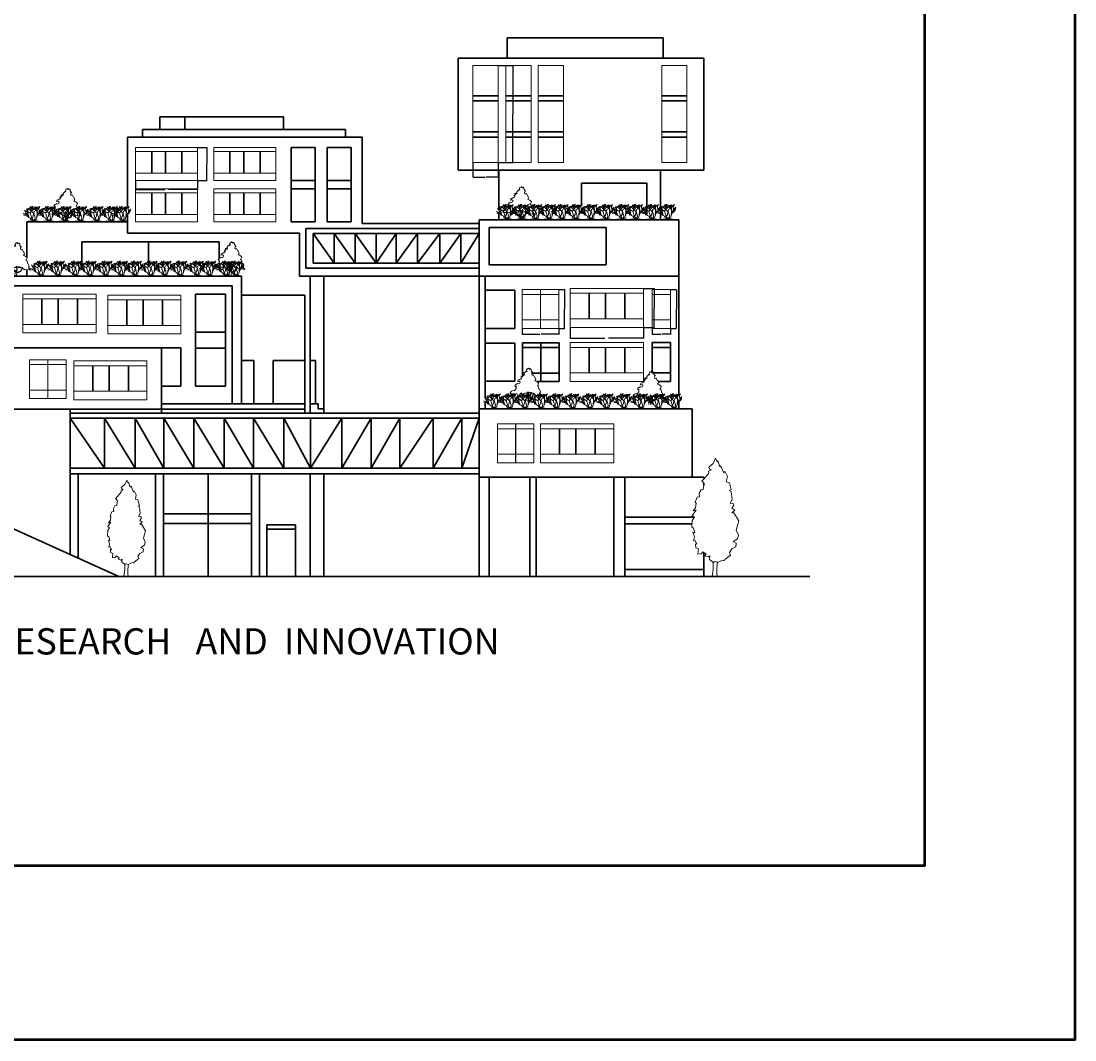
# Model space of a CAD drawing. Units: inches. Extents: x -1080 to 1950, y -1929 to 857.
# Tile 7 of 16: x 991 to 1950, y -1929 to -1001. Entities that reach past the tile are written whole.
import ezdxf

# ---------------------------------------------------------------- set-up
doc = ezdxf.new("R2010")
doc.units = ezdxf.units.IN
doc.header["$MEASUREMENT"] = 0
for name, color, linetype, lineweight in [('A-ANNO-DIMS', 2, 'Continuous', 18), ('A-ANNO-TEXT', 7, 'Continuous', 25), ('A-ANNO-TTLB', 7, 'Continuous', 50), ('A-ELEV', 7, 'Continuous', 35), ('A-GLAZ', 4, 'Continuous', 18), ('L-PLNT', 82, 'Continuous', 13)]:
    doc.layers.add(name, color=color, linetype=linetype, lineweight=lineweight)
doc.styles.get("Standard").update_dxf_attribs({"font": 'arial.ttf'})
doc.dimstyles.get("Standard").update_dxf_attribs({"dimtxt": 0.18, "dimasz": 0.18, "dimexe": 0.18, "dimexo": 0.0625, "dimgap": 0.09, "dimtad": 0, "dimtih": 1, "dimtoh": 1, "dimdec": 4, "dimzin": 0, "dimdsep": 46, "dimtxsty": 'Standard', "dimcen": 0.09, "dimadec": 0, "dimazin": 0, "dimtfac": 1, "dimtdec": 4, "dimtofl": 0, "dimtmove": 0, "dimatfit": 3, "dimfxl": 1, "dimtolj": 1, "dimtzin": 0, "dimarcsym": 0})

# ---------------------------------------------------------------- blocks, each defined once
blk = doc.blocks.new('*U5')
blk.add_lwpolyline([(-2.754, 191.699), (-6.78, 182.851), (-13.682, 176.953), (-11.956, 173.266), (-9.656, 172.529), (-14.257, 170.317), (-13.682, 167.368), (-21.733, 157.783), (-25.184, 154.834), (-21.158, 150.41), (-21.733, 147.461), (-22.884, 140.825), (-26.334, 140.087), (-29.21, 134.926), (-28.635, 129.028), (-32.661, 128.291), (-36.111, 120.18), (-34.386, 118.706), (-35.536, 111.333), (-38.987, 106.171), (-34.386, 107.646), (-40.712, 98.798), (-37.261, 95.849), (-40.712, 90.688), (-41.287, 80.366), (-38.412, 78.154), (-36.686, 70.781), (-39.562, 71.518), (-37.261, 64.145), (-38.412, 57.509), (-36.111, 58.247), (-33.236, 52.348), (-35.536, 53.086), (-34.961, 46.45), (-30.36, 44.975), (-31.51, 36.128), (-26.334, 36.865), (-23.459, 39.814), (-18.283, 36.128), (-20.008, 33.178), (-14.832, 31.704), (-11.956, 33.178), (-12.531, 27.28), (-6.205, 22.856), (-3.905, 24.331), (0.121, 22.856), (8.173, 26.543), (11.624, 25.068), (12.199, 27.28), (21.4, 34.653), (19.675, 39.077), (23.701, 44.975), (30.027, 47.924), (30.602, 53.823), (25.426, 56.772), (32.903, 61.196), (34.053, 67.094), (30.602, 75.205), (34.628, 89.951), (26.576, 103.222), (23.701, 103.222), (28.302, 107.646), (23.701, 110.595), (26.576, 115.756), (25.426, 117.968), (20.825, 118.706), (24.276, 124.604), (22.551, 137.876), (19.1, 139.35), (22.551, 140.825), (19.675, 151.884), (14.499, 153.359), (16.224, 162.207), (12.199, 170.317), (10.473, 167.368), (5.872, 179.165), (4.147, 177.69), (0.696, 187.275), (-0.454, 185.8)], close=True)
for points in [[(-6.813, 23.669), (-6.813, 11.669), (-8.627, 0)], [(0.387, 23.669), (-0.576, 13.271), (-0.576, 3.686), (0, 0)]]:
    blk.add_lwpolyline(points)
blk = doc.blocks.new('*U2')
for points in [[(22.0124, 137.721), (18.5475, 141.5624), (15.5282, 138.2446), (13.8028, 139.3505), (13.3714, 142.1153), (11.2148, 143.2214), (8.1954, 140.4564), (4.7447, 141.0094), (2.1567, 136.0326), (2.1567, 131.6088), (5.6074, 129.9499), (3.0193, 128.2909), (0.4313, 130.5029), (-6.9015, 123.3141), (-6.9015, 121.6552), (-9.9208, 119.9963), (-9.0581, 118.3373), (-6.9015, 115.0195), (-10.7835, 112.2546), (-14.6656, 115.0195), (-16.8222, 114.4665), (-17.6849, 112.2546), (-14.6656, 111.7016), (-14.2342, 107.2778), (-17.6065, 107.8307), (-21.5669, 103.9599), (-17.2536, 103.4069), (-18.9789, 97.8771), (-22.8609, 97.3241), (-27.1743, 94.5593), (-32.3504, 91.7944), (-32.7817, 94.0063), (-36.6638, 85.7116), (-29.7624, 87.3705), (-25.449, 84.6056), (-26.743, 77.9699), (-34.507, 75.205), (-37.9578, 77.4169), (-39.2518, 74.099), (-42.2711, 73.5461), (-44.8592, 70.2282), (-47.8786, 66.3574), (-43.9965, 63.0395), (-41.4085, 64.6985), (-44.3346, 59.8898), (-42.2089, 60.1377), (-42.5159, 55.7849), (-49.6039, 46.4502), (-58.2307, 45.8972), (-62.1127, 43.6853), (-68.5828, 36.4966), (-65.9947, 32.0727), (-50.0352, 32.6257), (-47.0159, 30.4138), (-39.6831, 33.7317), (-34.507, 22.6721), (-32.3504, 22.6721), (-22.4296, 34.8376), (-19.4102, 36.4966), (-17.2536, 33.7317), (-17.2536, 29.8608), (-13.8028, 28.7549), (-9.0581, 28.7549), (-7.3328, 32.6257), (-1.7254, 35.3906), (3.8821, 35.9436), (6.4701, 38.1555), (6.9014, 38.7085), (8.1954, 41.4734), (9.9208, 40.3674), (11.2148, 35.9436), (14.2341, 37.6025), (15.0968, 36.4966), (15.9595, 33.7317), (18.9789, 38.7085), (21.9982, 38.7085), (23.2922, 36.4966), (21.9982, 34.2847), (25.4489, 35.3906), (26.743, 33.7317), (29.7623, 35.9436), (32.7817, 34.8376), (38.8204, 28.7549), (41.4084, 27.6489), (43.5651, 25.437), (61.6813, 27.0959), (65.132, 23.7781), (67.7201, 24.884), (60.8186, 33.7317), (60.3873, 37.0495), (62.544, 40.3674), (58.662, 50.874), (56.5053, 50.874), (52.1919, 66.3574), (47.8785, 66.9103), (50.4665, 69.1222), (53.9172, 77.9699), (47.0158, 85.1586), (38.3891, 87.9235), (42.2711, 94.0063)], [(42.2711, 94.0063), (38.8204, 104.5129), (36.6637, 104.5129), (32.3503, 113.9135), (29.7623, 113.3605), (26.743, 113.3605), (24.5862, 117.7844), (25.8802, 123.8671), (29.331, 123.8671), (22.8609, 131.6088), (21.9982, 137.6916)], [(-12.9401, 28.7549), (-2.588, 22.1191), (0.8626, 17.6953), (1.7253, 11.6125), (0, 0)], [(-9.9208, 28.2019), (0, 23.2251), (3.4507, 19.9072), (4.7447, 15.4834), (8.6267, 27.0959), (6.4701, 37.6025)], [(34.5071, 33.1787), (27.1743, 18.2483), (9.0581, 10.5066), (7.7641, 3.8708), (8.1954, 0)], [(8.1954, 40.3674), (11.2148, 27.6489), (8.1954, 13.8245), (24.5862, 19.9072), (32.7817, 34.2847)]]:
    blk.add_lwpolyline(points)
blk = doc.blocks.new('*U6')
for p, q in [((-463.296, 280.416), (-552.577, 423.037)), ((-329.184, 316.992), (-499.872, 414.528)), ((-426.72, 414.528), (-475.488, 475.488)), ((-377.952, 463.296), (-451.104, 487.68)), ((-426.72, 414.528), (-390.144, 499.872)), ((-426.72, 316.992), (-426.72, 414.528)), ((-377.952, 463.296), (-329.184, 524.256)), ((-207.264, 304.8), (-377.952, 463.296)), ((-338.455, 424.7896), (-290.3982, 464.5406)), ((-329.184, 316.992), (-207.264, 451.104)), ((-316.7634, 502.285), (-327.6092, 559.9176)), ((-296.5958, 484.4034), (-316.7634, 502.285)), ((-286.512, 498.3226), (-307.4416, 538.0736)), ((-305.8922, 396.9512), (-302.7934, 478.4344)), ((-304.3428, 426.7708), (-268.7066, 458.5716)), ((-302.7934, 478.4344), (-270.256, 518.1854)), ((-290.3982, 464.5406), (-265.6078, 577.8246)), ((-268.7066, 458.5716), (-250.0884, 500.3038)), ((-207.264, 451.104), (-268.224, 548.64)), ((-240.792, 502.285), (-228.3968, 573.8368)), ((-182.88, 499.872), (-219.456, 512.064)), ((-207.264, 451.104), (-134.112, 487.68)), ((-182.88, 499.872), (-158.496, 536.448)), ((-121.92, 414.528), (-182.88, 499.872)), ((-182.88, 377.952), (-97.536, 426.72)), ((-129.1844, 450.6214), (-140.0302, 542.036)), ((-134.112, 487.68), (-97.536, 548.64)), ((-85.7758, 389.001), (-129.1844, 452.6026)), ((-73.152, 329.184), (-109.728, 499.872)), ((-97.536, 426.72), (-24.384, 524.256)), ((-85.7758, 472.4908), (-73.3552, 548.005)), ((-70.2564, 426.7708), (-85.7758, 472.4908)), ((-73.152, 402.336), (-60.96, 512.064)), ((-24.384, 268.224), (-73.152, 402.336)), ((-12.9032, 555.9552), (-2.0574, 522.1732)), ((-5.1562, 486.3846), (2.5908, 542.036)), ((8.7884, 335.3562), (-5.1562, 486.3846)), ((-3.6068, 492.3536), (14.986, 518.1854)), ((-0.508, 508.254), (22.7584, 536.067)), ((1.0414, 526.1356), (35.1536, 559.9176)), ((2.5908, 542.036), (21.209, 555.9552)), ((8.7884, 335.3562), (33.6042, 412.8516)), ((33.6042, 412.8516), (92.5068, 464.5406)), ((36.576, 390.144), (73.152, 438.912)), ((60.96, 390.144), (85.344, 414.528)), ((-451.104, 219.456), (-601.0402, 303.8094)), ((-451.104, 219.456), (-587.4512, 234.2388)), ((-463.296, 280.416), (-512.064, 292.608)), ((-353.568, 316.992), (-487.68, 377.952)), ((-402.336, 207.264), (-463.296, 280.416)), ((-414.528, 182.88), (-463.296, 182.88)), ((-426.72, 316.992), (-451.104, 329.184)), ((-377.952, 146.304), (-451.104, 219.456)), ((-402.336, 12.192), (-451.104, 0)), ((-402.336, 207.264), (-426.72, 316.992)), ((-377.952, 146.304), (-402.336, 207.264)), ((-341.376, 12.192), (-402.336, 12.192)), ((-329.184, 121.92), (-377.952, 146.304)), ((-329.184, 316.992), (-353.568, 316.992)), ((-243.84, 24.384), (-341.376, 12.192)), ((-268.224, 109.728), (-329.184, 316.992)), ((-292.608, 60.96), (-329.184, 121.92)), ((-243.84, 24.384), (-329.184, 0)), ((-219.456, 24.384), (-292.608, 60.96)), ((-268.224, 109.728), (-219.456, 195.072)), ((-219.456, 48.768), (-268.224, 109.728)), ((-243.84, 24.384), (-195.072, 24.384)), ((-219.456, 195.072), (-207.264, 304.8)), ((-219.456, 24.384), (-109.728, 73.152)), ((-219.456, 24.384), (-158.496, 73.152)), ((-219.456, 24.384), (-219.456, 48.768)), ((-219.456, 24.384), (-73.152, 24.384)), ((-195.072, 316.992), (-182.88, 377.952)), ((-170.688, 219.456), (-195.072, 316.992)), ((-195.072, 24.384), (-158.496, 12.192)), ((-146.304, 134.112), (-170.688, 219.456)), ((-158.496, 73.152), (-146.304, 134.112)), ((-158.496, 12.192), (-85.344, 0)), ((-109.728, 73.152), (-48.768, 243.84)), ((-85.344, 134.112), (-73.152, 329.184)), ((-73.152, 24.384), (0, 0)), ((-48.768, 243.84), (24.384, 304.8)), ((-12.192, 274.32), (8.7884, 335.3562)), ((24.384, 304.8), (36.576, 390.144)), ((24.384, 304.8), (73.152, 377.952)), ((48.768, 341.376), (60.96, 390.144))]:
    blk.add_line(p, q)
blk = doc.blocks.new('*U4')
for points in [[(559.11496, 3498.1134), (471.1065, 3595.68496), (394.41628, 3511.41284), (350.59112, 3539.5027), (339.63356, 3609.72862), (284.85592, 3637.82356), (208.16316, 3567.59256), (120.51538, 3581.63876), (54.78018, 3455.22804), (54.78018, 3342.86352), (142.42796, 3300.72746), (76.69022, 3258.58886), (10.95502, 3314.77366), (-175.2981, 3132.17814), (-175.2981, 3090.04208), (-251.98832, 3047.90602), (-230.07574, 3005.76742), (-175.2981, 2921.4953), (-273.9009, 2851.26684), (-372.50624, 2921.4953), (-427.28388, 2907.4491), (-449.19646, 2851.26684), (-372.50624, 2837.22064), (-361.54868, 2724.85612), (-447.2051, 2738.89978), (-547.79926, 2640.58146), (-438.24144, 2626.53526), (-482.06406, 2486.07834), (-580.66686, 2472.03214), (-690.22722, 2401.80622), (-821.70016, 2331.57776), (-832.65518, 2387.76002), (-931.26052, 2177.07464), (-755.96496, 2219.2107), (-646.4046, 2148.98224), (-679.2722, 1980.43546), (-876.4778, 1910.207), (-964.12812, 1966.38926), (-996.99572, 1882.1146), (-1073.68594, 1868.07094), (-1139.42368, 1783.79628), (-1216.11644, 1685.47796), (-1117.5111, 1601.2033), (-1051.7759, 1643.3419), (-1126.09884, 1521.20092), (-1072.10606, 1527.49758), (-1079.90386, 1416.93646), (-1259.93906, 1179.83508), (-1479.05978, 1165.78888), (-1577.66258, 1109.60662), (-1742.00312, 927.01364), (-1676.26538, 814.64658), (-1270.89408, 828.69278), (-1194.20386, 772.51052), (-1007.95074, 856.78518), (-876.4778, 575.87134), (-821.70016, 575.87134), (-569.71184, 884.87504), (-493.01908, 927.01364), (-438.24144, 856.78518), (-438.24144, 758.46432), (-350.59112, 730.37446), (-230.07574, 730.37446), (-186.25312, 828.69278), (-43.82516, 898.92124), (98.60534, 912.96744), (164.34054, 969.1497), (175.29556, 983.1959), (208.16316, 1053.42436), (251.98832, 1025.33196), (284.85592, 912.96744), (361.54614, 955.1035), (383.45872, 927.01364), (405.3713, 856.78518), (482.06406, 983.1959), (558.75428, 983.1959), (591.62188, 927.01364), (558.75428, 870.83138), (646.40206, 898.92124), (679.2722, 856.78518), (755.96242, 912.96744), (832.65518, 884.87504), (986.03816, 730.37446), (1051.77336, 702.28206), (1106.55354, 646.0998), (1566.70502, 688.23586), (1654.3528, 603.96374), (1720.09054, 632.0536), (1544.79244, 856.78518), (1533.83742, 941.0573), (1588.6176, 1025.33196), (1490.0148, 1292.1996), (1435.23462, 1292.1996), (1325.67426, 1685.47796), (1216.1139, 1699.52162), (1281.8491, 1755.70388), (1369.49688, 1980.43546), (1194.20132, 2163.02844), (975.08314, 2233.2569), (1073.68594, 2387.76002)], [(1073.68594, 2387.76002), (986.03816, 2654.62766), (931.25798, 2654.62766), (821.69762, 2893.4029), (755.96242, 2879.3567), (679.2722, 2879.3567), (624.48948, 2991.72376), (657.35708, 3146.22434), (745.0074, 3146.22434), (580.66686, 3342.86352), (558.75428, 3497.36664)], [(-328.67854, 730.37446), (-65.7352, 561.82514), (21.91004, 449.46062), (43.82262, 294.9575), (0, 0)], [(-251.98832, 716.32826), (0, 589.91754), (87.64778, 505.64288), (120.51538, 393.27836), (219.11818, 688.23586), (164.34054, 955.1035)], [(876.48034, 842.73898), (690.22722, 463.50682), (230.07574, 266.86764), (197.20814, 98.31832), (208.16316, 0)], [(208.16316, 1025.33196), (284.85592, 702.28206), (208.16316, 351.1423), (624.48948, 505.64288), (832.65518, 870.83138)]]:
    blk.add_lwpolyline(points)
blk = doc.blocks.new('WIN-TYPE-F')
for p, q in [((16.74, 35.39), (0, 35.39)), ((0, 35.39), (0, 31)), ((0, 31), (0, 7.71)), ((0, 31), (16.74, 31)), ((33.32, 35.39), (16.58, 35.39)), ((16.58, 35.39), (16.58, 31)), ((16.58, 31), (16.58, 7.71)), ((16.58, 31), (33.32, 31)), ((16.74, 35.39), (16.74, 31)), ((16.74, 7.71), (16.74, 31)), ((33.32, 35.39), (33.32, 31)), ((33.32, 7.71), (33.32, 31)), ((0, 7.71), (16.74, 7.71)), ((0, 7.71), (0, 0)), ((0, 0), (16.74, 0)), ((16.58, 7.71), (33.32, 7.71)), ((16.58, 7.71), (16.58, 0)), ((16.58, 0), (33.32, 0)), ((16.74, 0), (16.74, 7.71)), ((33.32, 0), (33.32, 7.71))]:
    blk.add_line(p, q)
blk = doc.blocks.new('WIN-TYPE-K')
for p, q in [((16.74, 35.39), (0, 35.39)), ((0, 35.39), (0, 31)), ((0, 31), (0, 7.71)), ((0, 31), (16.74, 31)), ((16.74, 35.39), (16.74, 31)), ((16.74, 7.71), (16.74, 31)), ((0, 7.71), (16.74, 7.71)), ((0, 7.71), (0, 0)), ((0, 0), (16.74, 0)), ((16.74, 0), (16.74, 7.71))]:
    blk.add_line(p, q)
blk = doc.blocks.new('WIN-TYPE-L')
for p, q in [((0, 31), (0, 35.39)), ((0, 35.39), (66.68, 35.39)), ((0, 31), (0, 7.71)), ((66.68, 31), (0, 31)), ((66.68, 35.39), (66.68, 31)), ((66.68, 7.71), (66.68, 31)), ((0, 7.71), (66.68, 7.71)), ((0, 7.71), (0, 0)), ((66.68, 0), (66.68, 7.71)), ((0, 0), (66.68, 0))]:
    blk.add_line(p, q)
blk = doc.blocks.new('WIN-TYPE-M')
for p, q in [((0, 26.24), (0, 29.96)), ((0, 29.96), (56.44, 29.96)), ((56.44, 29.96), (56.44, 26.24)), ((0, 26.24), (0, 6.52)), ((56.44, 26.24), (0, 26.24)), ((56.44, 6.52), (56.44, 26.24)), ((0, 6.52), (56.44, 6.52)), ((0, 6.52), (0, 0)), ((56.44, 0), (56.44, 6.52)), ((0, 0), (56.44, 0))]:
    blk.add_line(p, q)
blk = doc.blocks.new('PANEL-D')
for p, q in [((0, 88.25), (0, 0)), ((23.04, 88.25), (0, 88.25)), ((23.04, 0), (23.04, 88.25)), ((0, 0), (23.04, 0))]:
    blk.add_line(p, q)
blk = doc.blocks.new('*D45')
at = {"layer": 'A-ANNO-DIMS', "color": 0, "lineweight": -2, "transparency": 16777216}
for p, q in [((1480.39, -1245.41), (1485.82, -1245.41)), ((1485.64, -1245.59), (1485.64, -1262.92)), ((1485.64, -1280.62), (1485.64, -1263.29)), ((1480.39, -1280.8), (1485.82, -1280.8))]:
    blk.add_line(p, q, dxfattribs=at)
at = {"layer": 'A-ANNO-DIMS', "color": 0, "transparency": 16777216}
for points in [[(1485.61, -1245.59), (1485.67, -1245.59), (1485.64, -1245.41)], [(1485.61, -1280.62), (1485.67, -1280.62), (1485.64, -1280.8)]]:
    blk.add_solid(points, dxfattribs=at)
at = {"layer": 'Defpoints', "color": 0, "transparency": 16777216}
for p in [(1480.33, -1245.41), (1485.64, -1245.41), (1480.33, -1280.8)]:
    blk.add_point(p, dxfattribs=at)
at = {"layer": 'A-ANNO-DIMS', "color": 0, "transparency": 16777216, "insert": (1485.64, -1263.11), "char_height": 0.18, "attachment_point": 5}
blk.add_mtext('\\A1;WINDOW TYPE F 35 TYP.', dxfattribs=at)
blk = doc.blocks.new('*D46')
at = {"layer": 'A-ANNO-DIMS', "color": 0, "lineweight": -2, "transparency": 16777216}
for p, q in [((1447.01, -1280.86), (1447.01, -1286.29)), ((1447.19, -1286.11), (1463.14, -1286.11)), ((1480.15, -1286.11), (1464.2, -1286.11)), ((1480.33, -1280.86), (1480.33, -1286.29))]:
    blk.add_line(p, q, dxfattribs=at)
at = {"layer": 'A-ANNO-DIMS', "color": 0, "transparency": 16777216}
for points in [[(1447.19, -1286.08), (1447.19, -1286.14), (1447.01, -1286.11)], [(1480.15, -1286.08), (1480.15, -1286.14), (1480.33, -1286.11)]]:
    blk.add_solid(points, dxfattribs=at)
at = {"layer": 'Defpoints', "color": 0, "transparency": 16777216}
for p in [(1447.01, -1280.8), (1480.33, -1280.8), (1480.33, -1286.11)]:
    blk.add_point(p, dxfattribs=at)
at = {"layer": 'A-ANNO-DIMS', "color": 0, "transparency": 16777216, "insert": (1463.67, -1286.11), "char_height": 0.18, "attachment_point": 5}
blk.add_mtext('\\A1;33 TYP.', dxfattribs=at)
blk = doc.blocks.new('*D53')
at = {"layer": 'A-ANNO-DIMS', "color": 0, "lineweight": -2, "transparency": 16777216}
for p, q in [((1582.2, -1245.41), (1587.63, -1245.41)), ((1587.45, -1245.59), (1587.45, -1262.92)), ((1587.45, -1280.62), (1587.45, -1263.29)), ((1582.2, -1280.8), (1587.63, -1280.8))]:
    blk.add_line(p, q, dxfattribs=at)
at = {"layer": 'A-ANNO-DIMS', "color": 0, "transparency": 16777216}
for points in [[(1587.42, -1245.59), (1587.48, -1245.59), (1587.45, -1245.41)], [(1587.42, -1280.62), (1587.48, -1280.62), (1587.45, -1280.8)]]:
    blk.add_solid(points, dxfattribs=at)
at = {"layer": 'Defpoints', "color": 0, "transparency": 16777216}
for p in [(1582.14, -1245.41), (1587.45, -1245.41), (1582.14, -1280.8)]:
    blk.add_point(p, dxfattribs=at)
at = {"layer": 'A-ANNO-DIMS', "color": 0, "transparency": 16777216, "insert": (1587.45, -1263.11), "char_height": 0.18, "attachment_point": 5}
blk.add_mtext('\\A1;WINDOW TYPE K 35 TYP.', dxfattribs=at)
blk = doc.blocks.new('*D54')
at = {"layer": 'A-ANNO-DIMS', "color": 0, "lineweight": -2, "transparency": 16777216}
for p, q in [((1565.4, -1280.86), (1565.4, -1286.29)), ((1565.58, -1286.11), (1573.25, -1286.11)), ((1581.96, -1286.11), (1574.29, -1286.11)), ((1582.14, -1280.86), (1582.14, -1286.29))]:
    blk.add_line(p, q, dxfattribs=at)
at = {"layer": 'A-ANNO-DIMS', "color": 0, "transparency": 16777216}
for points in [[(1565.58, -1286.08), (1565.58, -1286.14), (1565.4, -1286.11)], [(1581.96, -1286.08), (1581.96, -1286.14), (1582.14, -1286.11)]]:
    blk.add_solid(points, dxfattribs=at)
at = {"layer": 'Defpoints', "color": 0, "transparency": 16777216}
for p in [(1565.4, -1280.8), (1582.14, -1280.8), (1582.14, -1286.11)]:
    blk.add_point(p, dxfattribs=at)
at = {"layer": 'A-ANNO-DIMS', "color": 0, "transparency": 16777216, "insert": (1573.77, -1286.11), "char_height": 0.18, "attachment_point": 5}
blk.add_mtext('\\A1;17 TYP.', dxfattribs=at)
blk = doc.blocks.new('*D55')
at = {"layer": 'A-ANNO-DIMS', "color": 0, "lineweight": -2, "transparency": 16777216}
for p, q in [((1490.64, -1279.91), (1490.64, -1290.03)), ((1557.32, -1279.91), (1557.32, -1290.03)), ((1490.82, -1289.85), (1522.39, -1289.85)), ((1557.14, -1289.85), (1525.57, -1289.85))]:
    blk.add_line(p, q, dxfattribs=at)
at = {"layer": 'A-ANNO-DIMS', "color": 0, "transparency": 16777216}
for points in [[(1490.82, -1289.82), (1490.82, -1289.88), (1490.64, -1289.85)], [(1557.14, -1289.82), (1557.14, -1289.88), (1557.32, -1289.85)]]:
    blk.add_solid(points, dxfattribs=at)
at = {"layer": 'Defpoints', "color": 0, "transparency": 16777216}
for p in [(1490.64, -1279.85), (1557.32, -1279.85), (1557.32, -1289.85)]:
    blk.add_point(p, dxfattribs=at)
at = {"layer": 'A-ANNO-DIMS', "color": 0, "transparency": 16777216, "insert": (1523.98, -1289.85), "char_height": 0.18, "attachment_point": 5}
blk.add_mtext('\\A1;WINDOW TYPE L 67 TYP.', dxfattribs=at)
blk = doc.blocks.new('*D56')
at = {"layer": 'A-ANNO-DIMS', "color": 0, "lineweight": -2, "transparency": 16777216}
for p, q in [((1557.38, -1244.46), (1567.5, -1244.46)), ((1567.32, -1244.64), (1567.32, -1261.97)), ((1567.32, -1279.67), (1567.32, -1262.33)), ((1557.38, -1279.85), (1567.5, -1279.85))]:
    blk.add_line(p, q, dxfattribs=at)
at = {"layer": 'A-ANNO-DIMS', "color": 0, "transparency": 16777216}
for points in [[(1567.29, -1244.64), (1567.35, -1244.64), (1567.32, -1244.46)], [(1567.29, -1279.67), (1567.35, -1279.67), (1567.32, -1279.85)]]:
    blk.add_solid(points, dxfattribs=at)
at = {"layer": 'Defpoints', "color": 0, "transparency": 16777216}
for p in [(1557.32, -1244.46), (1567.32, -1244.46), (1557.32, -1279.85)]:
    blk.add_point(p, dxfattribs=at)
at = {"layer": 'A-ANNO-DIMS', "color": 0, "transparency": 16777216, "insert": (1567.32, -1262.15), "char_height": 0.18, "attachment_point": 5}
blk.add_mtext('\\A1;35 TYP.', dxfattribs=at)
blk = doc.blocks.new('*D57')
at = {"layer": 'A-ANNO-DIMS', "color": 0, "lineweight": -2, "transparency": 16777216}
for p, q in [((1094.82, -1146.01), (1094.82, -1154.6)), ((1151.26, -1146.01), (1151.26, -1154.6)), ((1095, -1154.42), (1121.42, -1154.42)), ((1151.08, -1154.42), (1124.66, -1154.42))]:
    blk.add_line(p, q, dxfattribs=at)
at = {"layer": 'A-ANNO-DIMS', "color": 0, "transparency": 16777216}
for points in [[(1095, -1154.39), (1095, -1154.45), (1094.82, -1154.42)], [(1151.08, -1154.39), (1151.08, -1154.45), (1151.26, -1154.42)]]:
    blk.add_solid(points, dxfattribs=at)
at = {"layer": 'Defpoints', "color": 0, "transparency": 16777216}
for p in [(1094.82, -1145.95), (1151.26, -1145.95), (1151.26, -1154.42)]:
    blk.add_point(p, dxfattribs=at)
at = {"layer": 'A-ANNO-DIMS', "color": 0, "transparency": 16777216, "insert": (1123.04, -1154.42), "char_height": 0.18, "attachment_point": 5}
blk.add_mtext('\\A1;WINDOW TYPE M 56 TYP.', dxfattribs=at)
blk = doc.blocks.new('*D58')
at = {"layer": 'A-ANNO-DIMS', "color": 0, "lineweight": -2, "transparency": 16777216}
for p, q in [((1151.32, -1116), (1159.91, -1116)), ((1159.73, -1116.18), (1159.73, -1130.79)), ((1159.73, -1145.77), (1159.73, -1131.16)), ((1151.32, -1145.95), (1159.91, -1145.95))]:
    blk.add_line(p, q, dxfattribs=at)
at = {"layer": 'A-ANNO-DIMS', "color": 0, "transparency": 16777216}
for points in [[(1159.7, -1116.18), (1159.76, -1116.18), (1159.73, -1116)], [(1159.7, -1145.77), (1159.76, -1145.77), (1159.73, -1145.95)]]:
    blk.add_solid(points, dxfattribs=at)
at = {"layer": 'Defpoints', "color": 0, "transparency": 16777216}
for p in [(1151.26, -1116), (1159.73, -1116), (1151.26, -1145.95)]:
    blk.add_point(p, dxfattribs=at)
at = {"layer": 'A-ANNO-DIMS', "color": 0, "transparency": 16777216, "insert": (1159.73, -1130.97), "char_height": 0.18, "attachment_point": 5}
blk.add_mtext('\\A1;30 TYP.', dxfattribs=at)
blk = doc.blocks.new('*D77')
at = {"layer": 'A-ANNO-DIMS', "color": 0, "lineweight": -2, "transparency": 16777216}
for p, q in [((1425.25, -1041.43), (1438.6, -1041.43)), ((1438.42, -1041.61), (1438.42, -1085.37)), ((1438.42, -1129.49), (1438.42, -1085.73)), ((1425.25, -1129.67), (1438.6, -1129.67))]:
    blk.add_line(p, q, dxfattribs=at)
at = {"layer": 'A-ANNO-DIMS', "color": 0, "transparency": 16777216}
for points in [[(1438.39, -1041.61), (1438.45, -1041.61), (1438.42, -1041.43)], [(1438.39, -1129.49), (1438.45, -1129.49), (1438.42, -1129.67)]]:
    blk.add_solid(points, dxfattribs=at)
at = {"layer": 'Defpoints', "color": 0, "transparency": 16777216}
for p in [(1425.19, -1041.43), (1438.42, -1041.43), (1425.19, -1129.67)]:
    blk.add_point(p, dxfattribs=at)
at = {"layer": 'A-ANNO-DIMS', "color": 0, "transparency": 16777216, "insert": (1438.42, -1085.55), "char_height": 0.18, "attachment_point": 5}
blk.add_mtext('\\A1;PANEL D 88 TYP.', dxfattribs=at)
blk = doc.blocks.new('*D78')
at = {"layer": 'A-ANNO-DIMS', "color": 0, "lineweight": -2, "transparency": 16777216}
for p, q in [((1402.15, -1129.74), (1402.15, -1143.09)), ((1425.19, -1129.74), (1425.19, -1143.09)), ((1402.33, -1142.91), (1413.14, -1142.91)), ((1425.01, -1142.91), (1414.2, -1142.91))]:
    blk.add_line(p, q, dxfattribs=at)
at = {"layer": 'A-ANNO-DIMS', "color": 0, "transparency": 16777216}
for points in [[(1402.33, -1142.88), (1402.33, -1142.94), (1402.15, -1142.91)], [(1425.01, -1142.88), (1425.01, -1142.94), (1425.19, -1142.91)]]:
    blk.add_solid(points, dxfattribs=at)
at = {"layer": 'Defpoints', "color": 0, "transparency": 16777216}
for p in [(1402.15, -1129.67), (1425.19, -1129.67), (1425.19, -1142.91)]:
    blk.add_point(p, dxfattribs=at)
at = {"layer": 'A-ANNO-DIMS', "color": 0, "transparency": 16777216, "insert": (1413.67, -1142.91), "char_height": 0.18, "attachment_point": 5}
blk.add_mtext('\\A1;23 TYP.', dxfattribs=at)

msp = doc.modelspace()

# ---------------------------------------------------------------- linework, layer by layer
at = {"layer": 'A-ANNO-TTLB'}
for points in [[(-1080.09, 856.52), (1950.41, 856.52), (1950.41, -1928.98), (-1080.09, -1928.98)], [(-957.59, 743.52), (1813.41, 743.52), (1813.41, -1770.48), (-957.59, -1770.48)]]:
    msp.add_lwpolyline(points, close=True, dxfattribs=at)
at = {"layer": 'A-ELEV'}
for p, q in [((1433.14, -1034.61), (1433.14, -1016.26)), ((1433.14, -1016.26), (1575.3, -1016.26)), ((1575.3, -1016.26), (1575.3, -1034.61)), ((1388.54, -1034.61), (1612.42, -1034.61)), ((1388.54, -1136.77), (1388.54, -1034.61)), ((1612.42, -1070.15), (1612.42, -1034.61)), ((1402.15, -1068.81), (1425.19, -1068.81)), ((1402.15, -1073.39), (1425.19, -1073.39)), ((1432.15, -1068.81), (1455.19, -1068.81)), ((1432.15, -1073.39), (1455.19, -1073.39)), ((1461.45, -1068.81), (1484.49, -1068.81)), ((1461.45, -1073.39), (1484.49, -1073.39)), ((1574.01, -1068.81), (1597.05, -1068.81)), ((1574.01, -1073.39), (1597.05, -1073.39)), ((1612.42, -1070.15), (1612.42, -1136.77)), ((1116.95, -1091.48), (1116.95, -1088.21)), ((1116.95, -1088.21), (1229.42, -1088.21)), ((1116.95, -1099.55), (1116.95, -1091.48)), ((1139.77, -1099.55), (1139.77, -1088.21)), ((1229.42, -1088.21), (1229.42, -1099.55)), ((1101.1, -1106.72), (1101.1, -1099.55)), ((1101.1, -1099.55), (1286.06, -1099.55)), ((1286.06, -1099.55), (1286.06, -1106.72)), ((1402.15, -1101.65), (1425.19, -1101.65)), ((1432.15, -1101.65), (1455.19, -1101.65)), ((1461.45, -1101.65), (1484.49, -1101.65)), ((1574.01, -1101.65), (1597.05, -1101.65)), ((1087.46, -1121.98), (1087.46, -1106.72)), ((1087.46, -1106.72), (1294.18, -1106.72)), ((1294.18, -1106.72), (1301.34, -1106.72)), ((1301.34, -1106.72), (1301.34, -1185.13)), ((1402.15, -1106.74), (1425.19, -1106.74)), ((1432.15, -1106.74), (1455.19, -1106.74)), ((1461.45, -1106.74), (1484.49, -1106.74)), ((1574.01, -1106.74), (1597.05, -1106.74)), ((1087.46, -1148.02), (1087.46, -1121.98)), ((1109.61, -1119.71), (1109.61, -1139.43)), ((1122.11, -1119.71), (1122.11, -1139.43)), ((1137.09, -1119.71), (1137.09, -1139.43)), ((1180.81, -1119.71), (1180.81, -1139.43)), ((1193.31, -1119.71), (1193.31, -1139.43)), ((1208.3, -1119.71), (1208.3, -1139.43)), ((1236.55, -1116), (1236.55, -1183.59)), ((1258.48, -1116), (1236.55, -1116)), ((1258.48, -1183.59), (1258.48, -1116)), ((1269.3, -1116), (1269.3, -1183.59)), ((1291.22, -1116), (1269.3, -1116)), ((1291.22, -1183.59), (1291.22, -1116)), ((1388.54, -1136.77), (1612.42, -1136.77)), ((1425.6, -1136.77), (1407.76, -1136.77)), ((1425.6, -1173.01), (1425.6, -1136.77)), ((1572.96, -1181.78), (1572.96, -1136.77)), ((1087.46, -1148.02), (1087.46, -1170.71)), ((1236.55, -1145.95), (1258.48, -1145.95)), ((1269.3, -1145.95), (1291.22, -1145.95)), ((1500.87, -1168.37), (1500.87, -1148.62)), ((1500.87, -1148.62), (1560.52, -1148.62)), ((1560.52, -1148.62), (1560.52, -1177.54)), ((1109.61, -1157.35), (1109.61, -1177.07)), ((1122.11, -1157.35), (1122.11, -1177.07)), ((1137.09, -1157.35), (1137.09, -1177.07)), ((1180.81, -1157.35), (1180.81, -1177.07)), ((1193.31, -1157.35), (1193.31, -1177.07)), ((1208.3, -1157.35), (1208.3, -1177.07)), ((1236.55, -1153.64), (1258.48, -1153.64)), ((1269.3, -1153.64), (1291.22, -1153.64)), ((1087.46, -1176.68), (1087.46, -1191.75)), ((1425.6, -1181.78), (1425.6, -1176.18)), ((1500.87, -1176.06), (1500.87, -1174.55)), ((1087.46, -1183.59), (995.74, -1183.59)), ((995.74, -1183.59), (995.74, -1216.11)), ((1236.55, -1183.59), (1258.48, -1183.59)), ((1407.76, -1189.84), (1249.95, -1189.84)), ((1249.95, -1226.04), (1249.95, -1189.84)), ((1269.3, -1183.59), (1291.22, -1183.59)), ((1301.34, -1185.13), (1407.76, -1185.13)), ((1407.76, -1181.78), (1407.76, -1197.38)), ((1407.76, -1181.78), (1589.78, -1181.78)), ((1523.51, -1188.76), (1416.84, -1188.76)), ((1416.84, -1188.76), (1416.84, -1223.02)), ((1523.51, -1223.02), (1523.51, -1188.76)), ((1560.52, -1181.37), (1560.52, -1181.78)), ((1589.78, -1233.27), (1589.78, -1181.78)), ((1589.78, -1181.78), (1589.78, -1184.14)), ((1589.78, -1181.78), (1589.78, -1341.35)), ((1087.46, -1194.1), (1087.46, -1191.75)), ((1244.12, -1194.1), (1087.46, -1194.1)), ((1244.12, -1194.1), (1244.12, -1226.04)), ((1256.64, -1194.48), (1407.76, -1194.48)), ((1256.64, -1194.48), (1256.64, -1221.49)), ((1256.64, -1194.48), (1275.77, -1221.49)), ((1275.77, -1194.48), (1275.77, -1221.49)), ((1275.77, -1194.48), (1294.81, -1221.49)), ((1294.81, -1194.48), (1294.81, -1221.49)), ((1294.81, -1194.48), (1314.04, -1221.49)), ((1314.04, -1194.48), (1314.04, -1221.49)), ((1314.04, -1221.49), (1332.13, -1194.48)), ((1332.13, -1194.48), (1332.13, -1221.49)), ((1351.56, -1194.48), (1332.13, -1221.49)), ((1351.56, -1194.48), (1351.56, -1221.49)), ((1371.93, -1194.48), (1351.56, -1221.49)), ((1371.93, -1194.48), (1371.93, -1221.49)), ((1391.17, -1194.48), (1371.93, -1221.49)), ((1391.17, -1194.48), (1391.17, -1221.49)), ((1407.76, -1194.48), (1391.17, -1221.49)), ((1407.76, -1233.27), (1407.76, -1197.38)), ((1046.01, -1222.83), (1046.01, -1201.97)), ((1046.01, -1201.97), (1170.88, -1201.97)), ((1106.57, -1201.97), (1106.57, -1224.59)), ((1170.88, -1201.97), (1170.88, -1217.2)), ((1407.76, -1229.03), (1407.76, -1202.02)), ((995.74, -1227.24), (995.74, -1233.27)), ((1046.01, -1227.72), (1046.01, -1224.83)), ((1244.12, -1226.04), (1244.12, -1233.27)), ((1249.95, -1226.04), (1407.76, -1226.04)), ((1256.64, -1221.49), (1407.76, -1221.49)), ((1416.84, -1223.02), (1523.51, -1223.02)), ((1191.24, -1233.27), (903.9, -1233.27)), ((1106.57, -1232.75), (1106.57, -1233.27)), ((1171.17, -1233.18), (1171.17, -1233.27)), ((1191.24, -1233.27), (1191.24, -1349.66)), ((1244.12, -1233.27), (1589.78, -1233.27)), ((1253.9, -1233.27), (1253.9, -1358.11)), ((1266.26, -1233.27), (1266.26, -1358.11)), ((1407.76, -1233.27), (1407.76, -1354.12)), ((1413.2, -1294.13), (1413.2, -1233.27)), ((1182.73, -1242), (977.91, -1242)), ((1182.73, -1242), (1182.73, -1349.66)), ((1413.2, -1246.09), (1440.4, -1246.09)), ((1413.2, -1280.8), (1413.2, -1246.09)), ((1440.4, -1246.09), (1440.4, -1280.8)), ((1009.58, -1253.99), (1009.58, -1277.29)), ((1024.34, -1253.99), (1024.34, -1277.29)), ((1042.05, -1253.99), (1042.05, -1277.29)), ((1086.9, -1254.86), (1086.9, -1278.16)), ((1101.67, -1254.86), (1101.67, -1278.16)), ((1119.37, -1254.86), (1119.37, -1278.16)), ((1149.45, -1249.57), (1176.65, -1249.57)), ((1149.45, -1284.29), (1149.45, -1249.57)), ((1176.65, -1249.57), (1176.65, -1284.29)), ((1191.24, -1250.64), (1249.06, -1250.64)), ((1249.06, -1250.64), (1249.06, -1358.11)), ((1508.11, -1248.85), (1508.11, -1272.14)), ((1522.88, -1248.85), (1522.88, -1272.14)), ((1540.58, -1248.85), (1540.58, -1272.14)), ((1176.65, -1284.29), (1149.45, -1284.29)), ((1149.45, -1284.29), (1149.45, -1298.78)), ((1176.65, -1284.29), (1176.65, -1298.78)), ((1440.4, -1280.8), (1413.2, -1280.8)), ((1413.2, -1294.13), (1440.4, -1294.13)), ((1413.2, -1328.84), (1413.2, -1294.13)), ((1440.4, -1294.13), (1440.4, -1328.84)), ((1464.06, -1293.94), (1447.32, -1293.94)), ((1447.32, -1293.94), (1447.32, -1298.33)), ((1480.64, -1293.94), (1463.91, -1293.94)), ((1463.91, -1293.94), (1463.91, -1298.33)), ((1464.06, -1293.94), (1464.06, -1298.33)), ((1480.64, -1293.94), (1480.64, -1298.33)), ((1582.14, -1293.71), (1565.4, -1293.71)), ((1565.4, -1293.71), (1565.4, -1298.1)), ((1582.14, -1293.71), (1582.14, -1298.1)), ((1118.58, -1298.48), (977.91, -1298.48)), ((1118.58, -1349.66), (1118.58, -1298.48)), ((1118.58, -1298.48), (1136.11, -1298.48)), ((1136.11, -1298.48), (1136.11, -1333.49)), ((1149.45, -1298.78), (1176.65, -1298.78)), ((1149.45, -1333.49), (1149.45, -1298.78)), ((1176.65, -1298.78), (1176.65, -1333.49)), ((1447.32, -1298.33), (1447.32, -1321.62)), ((1447.32, -1298.33), (1464.06, -1298.33)), ((1463.91, -1298.33), (1463.91, -1321.62)), ((1463.91, -1298.33), (1480.64, -1298.33)), ((1464.06, -1321.62), (1464.06, -1298.33)), ((1480.64, -1321.62), (1480.64, -1298.33)), ((1508.11, -1298.1), (1508.11, -1321.39)), ((1522.88, -1298.1), (1522.88, -1321.39)), ((1540.58, -1298.1), (1540.58, -1321.39)), ((1565.4, -1298.1), (1565.4, -1321.39)), ((1565.4, -1298.1), (1582.14, -1298.1)), ((1582.14, -1321.39), (1582.14, -1298.1)), ((1056.01, -1314.84), (1056.01, -1338.14)), ((1070.78, -1314.84), (1070.78, -1338.14)), ((1088.49, -1314.84), (1088.49, -1338.14)), ((1202.57, -1310.01), (1191.24, -1310.01)), ((1202.57, -1310.01), (1202.57, -1349.66)), ((1249.06, -1310.01), (1220.26, -1310.01)), ((1220.26, -1310.01), (1220.26, -1349.66)), ((1253.9, -1310.01), (1258.77, -1310.01)), ((1258.77, -1310.01), (1258.77, -1349.66)), ((1447.32, -1321.62), (1448.91, -1321.62)), ((1447.32, -1321.62), (1447.32, -1324.62)), ((1455.77, -1321.62), (1464.06, -1321.62)), ((1463.91, -1321.62), (1480.64, -1321.62)), ((1463.91, -1321.62), (1463.91, -1329.33)), ((1464.06, -1329.33), (1464.06, -1321.62)), ((1480.64, -1329.33), (1480.64, -1321.62)), ((1565.4, -1321.39), (1582.14, -1321.39)), ((1582.14, -1329.1), (1582.14, -1321.39)), ((1136.11, -1333.49), (1118.58, -1333.49)), ((1176.65, -1333.49), (1149.45, -1333.49)), ((1440.4, -1328.84), (1413.2, -1328.84)), ((1413.2, -1328.84), (1413.2, -1344.39)), ((1460.37, -1329.33), (1464.06, -1329.33)), ((1463.91, -1329.33), (1480.64, -1329.33)), ((1570.69, -1329.1), (1582.14, -1329.1)), ((1590.17, -1341.35), (1590.55, -1341.35)), ((1182.73, -1349.66), (1118.58, -1349.66)), ((1118.58, -1349.66), (1118.58, -1358.11)), ((1118.58, -1349.66), (1249.06, -1349.66)), ((1258.77, -1349.66), (1253.9, -1349.66)), ((1258.77, -1349.66), (1261.23, -1349.66)), ((1261.23, -1349.66), (1261.23, -1354.09)), ((1413.2, -1348.52), (1413.2, -1354.12)), ((1589.78, -1354.12), (1589.78, -1347.55)), ((1118.58, -1354.46), (982.83, -1354.46)), ((1035.23, -1358.11), (1035.23, -1354.46)), ((1118.58, -1358.11), (1035.23, -1358.11)), ((1035.23, -1362.7), (1035.23, -1358.11)), ((1118.58, -1362.7), (1035.23, -1362.7)), ((1035.23, -1362.7), (1035.23, -1480.68)), ((1035.23, -1362.7), (1066.59, -1408.03)), ((1066.59, -1362.7), (1066.59, -1408.03)), ((1066.59, -1362.7), (1094.55, -1408.03)), ((1094.55, -1362.7), (1094.55, -1408.03)), ((1094.55, -1362.7), (1120.48, -1408.03)), ((1118.58, -1354.46), (1249.06, -1354.46)), ((1118.58, -1358.11), (1253.9, -1358.11)), ((1272.31, -1362.7), (1118.58, -1362.7)), ((1120.48, -1362.7), (1120.48, -1408.03)), ((1120.48, -1362.7), (1147.76, -1408.03)), ((1147.76, -1362.7), (1147.76, -1408.03)), ((1147.76, -1362.7), (1175.53, -1408.03)), ((1175.53, -1362.7), (1175.53, -1408.03)), ((1175.53, -1362.7), (1202.2, -1408.03)), ((1277.21, -1358.11), (1191.24, -1358.11)), ((1202.2, -1362.7), (1202.2, -1408.03)), ((1202.2, -1362.7), (1229.84, -1408.03)), ((1229.84, -1362.7), (1229.84, -1408.03)), ((1229.84, -1362.7), (1254.3, -1408.03)), ((1254.3, -1362.7), (1254.3, -1408.03)), ((1282.67, -1362.7), (1254.3, -1408.03)), ((1261.23, -1354.09), (1266.26, -1354.09)), ((1407.76, -1362.7), (1272.31, -1362.7)), ((1277.21, -1358.11), (1407.76, -1358.11)), ((1282.67, -1362.7), (1282.67, -1408.03)), ((1309.34, -1362.7), (1282.67, -1408.03)), ((1309.34, -1362.7), (1309.34, -1408.03)), ((1335.46, -1362.7), (1309.34, -1408.03)), ((1335.46, -1362.7), (1335.46, -1408.03)), ((1365.99, -1362.7), (1335.46, -1408.03)), ((1365.99, -1362.7), (1365.99, -1408.03)), ((1391.92, -1362.7), (1365.99, -1408.03)), ((1391.92, -1362.7), (1391.92, -1408.03)), ((1407.76, -1362.7), (1391.92, -1408.03)), ((1407.76, -1354.12), (1589.78, -1354.12)), ((1407.76, -1354.12), (1407.76, -1416.44)), ((1589.78, -1354.13), (1601.86, -1354.13)), ((1601.86, -1354.13), (1601.86, -1416.44)), ((1481.09, -1372.18), (1481.09, -1395.48)), ((1495.86, -1372.18), (1495.86, -1395.48)), ((1513.57, -1372.18), (1513.57, -1395.48)), ((835.56, -1396.69), (1079.47, -1506.72)), ((1277.21, -1408.03), (1035.23, -1408.03)), ((1407.76, -1408.03), (1277.21, -1408.03)), ((1294.81, -1413.44), (1035.23, -1413.44)), ((1042.45, -1413.44), (1042.45, -1490.02)), ((1112.92, -1413.44), (1112.92, -1506.72)), ((1120.35, -1413.44), (1120.35, -1506.72)), ((1160.84, -1413.44), (1160.84, -1506.72)), ((1200.41, -1413.44), (1200.41, -1506.72)), ((1207.84, -1413.44), (1207.84, -1506.72)), ((1253.9, -1413.44), (1253.9, -1506.72)), ((1266.26, -1413.44), (1266.26, -1506.72)), ((1407.76, -1413.44), (1294.81, -1413.44)), ((1601.86, -1416.44), (1407.76, -1416.44)), ((1407.76, -1416.44), (1407.76, -1506.72)), ((1416.81, -1416.44), (1416.81, -1506.72)), ((1453.98, -1416.44), (1453.98, -1506.72)), ((1459.74, -1416.44), (1459.74, -1506.72)), ((1530.3, -1416.44), (1530.3, -1506.72)), ((1540.37, -1506.72), (1540.37, -1416.44)), ((1612.48, -1416.44), (1596.11, -1416.44)), ((1601.86, -1416.44), (1601.86, -1416.44)), ((1601.86, -1416.44), (1601.86, -1416.44)), ((1601.86, -1416.44), (1601.86, -1416.44)), ((1612.48, -1416.44), (1612.48, -1418.07)), ((1612.48, -1421.84), (1612.48, -1423.93)), ((1120.35, -1449.61), (1200.41, -1449.61)), ((1120.35, -1458.45), (1200.41, -1458.45)), ((1540.37, -1452.9), (1603.75, -1452.9)), ((1540.37, -1458.95), (1601.64, -1458.95)), ((1214.35, -1459.68), (1240.56, -1459.68)), ((1214.35, -1459.68), (1214.35, -1506.72)), ((1214.35, -1463.56), (1240.56, -1463.56)), ((1240.56, -1459.68), (1240.56, -1506.72)), ((1035.23, -1480.68), (1035.23, -1486.76)), ((1612.48, -1485.08), (1612.48, -1506.72)), ((1612.48, -1506.72), (332.83, -1506.72)), ((1540.37, -1500.36), (1612.48, -1500.36)), ((1612.48, -1506.72), (1708.83, -1506.72))]:
    msp.add_line(p, q, dxfattribs=at)

# ---------------------------------------------------------------- block references
at = {"layer": 'A-GLAZ'}
for name, p in [('PANEL-D', (1402.15, -1129.67)), ('PANEL-D', (1432.15, -1129.67)), ('PANEL-D', (1461.45, -1129.67)), ('PANEL-D', (1574.01, -1129.67)), ('WIN-TYPE-M', (1094.82, -1145.95)), ('WIN-TYPE-M', (1166.02, -1145.95)), ('WIN-TYPE-M', (1094.82, -1183.59)), ('WIN-TYPE-M', (1166.02, -1183.59)), ('WIN-TYPE-F', (1447.01, -1280.8)), ('WIN-TYPE-L', (1490.64, -1279.85)), ('WIN-TYPE-K', (1565.4, -1280.8)), ('WIN-TYPE-L', (992.1, -1284.99)), ('WIN-TYPE-L', (1069.42, -1285.86)), ('WIN-TYPE-L', (1490.64, -1329.1)), ('WIN-TYPE-F', (998.2, -1344.79)), ('WIN-TYPE-L', (1038.54, -1345.84)), ('WIN-TYPE-F', (1424.38, -1403.21)), ('WIN-TYPE-L', (1463.62, -1403.18))]:
    msp.add_blockref(name, p, dxfattribs=at)
at = {"layer": 'L-PLNT'}
for name, p, xscale, yscale, zscale in [('*U4', (1443.94, -1182.04), 0.0083091553795611, 0.0083091553795611, 0.0083091553795611), ('*U2', (1030.49, -1183.33), 0.2096355800251992, 0.2096355800251992, 0.2096355800251992), ('*U6', (1006.91, -1183.35), 0.024256363829807, 0.024256363829807, 0.024256363829807), ('*U6', (1020.85, -1183.35), 0.024256363829807, 0.024256363829807, 0.024256363829807), ('*U6', (1035.35, -1183.35), 0.024256363829807, 0.024256363829807, 0.024256363829807), ('*U6', (1049.48, -1183.35), 0.024256363829807, 0.024256363829807, 0.024256363829807), ('*U6', (1064.45, -1183.35), 0.024256363829807, 0.024256363829807, 0.024256363829807), ('*U6', (1077.54, -1183.35), 0.024256363829807, 0.024256363829807, 0.024256363829807), ('*U6', (1088.11, -1183.35), 0.024256363829807, 0.024256363829807, 0.024256363829807), ('*U6', (1438, -1181.66), 0.024256363829807, 0.024256363829807, 0.024256363829807), ('*U6', (1451.73, -1181.66), 0.024256363829807, 0.024256363829807, 0.024256363829807), ('*U6', (1464.04, -1181.66), 0.024256363829807, 0.024256363829807, 0.024256363829807), ('*U6', (1476.35, -1181.66), 0.024256363829807, 0.024256363829807, 0.024256363829807), ('*U6', (1488.03, -1181.66), 0.024256363829807, 0.024256363829807, 0.024256363829807), ('*U6', (1500.61, -1181.66), 0.024256363829807, 0.024256363829807, 0.024256363829807), ('*U6', (1514.42, -1181.66), 0.024256363829807, 0.024256363829807, 0.024256363829807), ('*U6', (1528.41, -1181.66), 0.024256363829807, 0.024256363829807, 0.024256363829807), ('*U6', (1543.21, -1181.66), 0.024256363829807, 0.024256363829807, 0.024256363829807), ('*U6', (1555.65, -1181.66), 0.024256363829807, 0.024256363829807, 0.024256363829807), ('*U6', (1570.26, -1181.66), 0.024256363829807, 0.024256363829807, 0.024256363829807), ('*U6', (1584.69, -1181.66), 0.024256363829807, 0.024256363829807, 0.024256363829807), ('*U2', (984.71, -1232.74), 0.2096355800251992, 0.2096355800251992, 0.2096355800251992), ('*U4', (1180.13, -1232.3), 0.0083091553795611, 0.0083091553795611, 0.0083091553795611), ('*U6', (1013.54, -1233.18), 0.024256363829807, 0.024256363829807, 0.024256363829807), ('*U6', (1029.11, -1233.18), 0.024256363829807, 0.024256363829807, 0.024256363829807), ('*U6', (1044.81, -1233.18), 0.024256363829807, 0.024256363829807, 0.024256363829807), ('*U6', (1058.18, -1233.18), 0.024256363829807, 0.024256363829807, 0.024256363829807), ('*U6', (1072.58, -1233.18), 0.024256363829807, 0.024256363829807, 0.024256363829807), ('*U6', (1086.75, -1233.18), 0.024256363829807, 0.024256363829807, 0.024256363829807), ('*U6', (1099.34, -1233.18), 0.024256363829807, 0.024256363829807, 0.024256363829807), ('*U6', (1113.74, -1233.18), 0.024256363829807, 0.024256363829807, 0.024256363829807), ('*U6', (1126.34, -1233.18), 0.024256363829807, 0.024256363829807, 0.024256363829807), ('*U6', (1140.51, -1233.18), 0.024256363829807, 0.024256363829807, 0.024256363829807), ('*U6', (1155.8, -1233.18), 0.024256363829807, 0.024256363829807, 0.024256363829807), ('*U6', (1167.05, -1233.18), 0.024256363829807, 0.024256363829807, 0.024256363829807), ('*U6', (1182.12, -1233.18), 0.024256363829807, 0.024256363829807, 0.024256363829807), ('*U6', (1191.19, -1233.18), 0.024256363829807, 0.024256363829807, 0.024256363829807), ('*U4', (1450.42, -1347.27), 0.0083091553795611, 0.0083091553795611, 0.0083091553795611), ('*U4', (1562.19, -1350.23), 0.0083091553795611, 0.0083091553795611, 0.0083091553795611), ('*U6', (1426.24, -1354.07), 0.024256363829807, 0.024256363829807, 0.024256363829807), ('*U6', (1440.42, -1354.07), 0.024256363829807, 0.024256363829807, 0.024256363829807), ('*U6', (1454.38, -1354.07), 0.024256363829807, 0.024256363829807, 0.024256363829807), ('*U6', (1469.07, -1354.07), 0.024256363829807, 0.024256363829807, 0.024256363829807), ('*U6', (1483.07, -1354.07), 0.024256363829807, 0.024256363829807, 0.024256363829807), ('*U6', (1497.77, -1354.07), 0.024256363829807, 0.024256363829807, 0.024256363829807), ('*U6', (1513.56, -1354.07), 0.024256363829807, 0.024256363829807, 0.024256363829807), ('*U6', (1528.84, -1354.07), 0.024256363829807, 0.024256363829807, 0.024256363829807), ('*U6', (1544.54, -1354.07), 0.024256363829807, 0.024256363829807, 0.024256363829807), ('*U6', (1560.16, -1354.07), 0.024256363829807, 0.024256363829807, 0.024256363829807), ('*U6', (1575.91, -1354.07), 0.024256363829807, 0.024256363829807, 0.024256363829807), ('*U6', (1590.24, -1354.07), 0.024256363829807, 0.024256363829807, 0.024256363829807), ('*U5', (1624.71, -1506.78), 0.5622556922993422, 0.5622556922993422, 0.5622556922993422), ('*U5', (1088.05, -1506.23), 0.4553241752017993, 0.4553241752017993, 0.4553241752017993)]:
    msp.add_blockref(name, p, dxfattribs=dict(at, xscale=xscale, yscale=yscale, zscale=zscale))

# ---------------------------------------------------------------- texts
at = {"layer": 'A-ANNO-TEXT'}
msp.add_text('LINEAR   CAMPUS   AXIS   ELEVATION   RESEARCH   AND  INNOVATION', height=23.9238, dxfattribs=at).set_placement((395.19, -1577.87))

# ---------------------------------------------------------------- dimensions: what is measured, and where the dimension line sits
at = {"layer": 'A-ANNO-DIMS'}
for base, p1, p2, text, picture, middle in [((1438.42, -1041.43), (1425.19, -1129.67), (1425.19, -1041.43), 'PANEL D <> TYP.', '*D77', (1438.42, -1085.55)), ((1159.73, -1116), (1151.26, -1145.95), (1151.26, -1116), '<> TYP.', '*D58', (1159.73, -1130.97)), ((1485.64, -1245.41), (1480.33, -1280.8), (1480.33, -1245.41), 'WINDOW TYPE F <> TYP.', '*D45', (1485.64, -1263.11)), ((1567.32, -1244.46), (1557.32, -1279.85), (1557.32, -1244.46), '<> TYP.', '*D56', (1567.32, -1262.15)), ((1587.45, -1245.41), (1582.14, -1280.8), (1582.14, -1245.41), 'WINDOW TYPE K <> TYP.', '*D53', (1587.45, -1263.11))]:
    dim = msp.add_linear_dim(base=base, p1=p1, p2=p2, angle=90, text=text, dimstyle='Standard', override={"dimdec": 0, "dimlfac": 1, "dimrnd": 0, "dimzin": 0, "dimdsep": 46, "dimlunit": 2}, dxfattribs=at)
    dim.commit()
    dim.dimension.update_dxf_attribs({"geometry": picture, "text_midpoint": middle})
for base, p1, p2, text, picture, middle in [((1425.19, -1142.91), (1402.15, -1129.67), (1425.19, -1129.67), '<> TYP.', '*D78', (1413.67, -1142.91)), ((1151.26, -1154.42), (1094.82, -1145.95), (1151.26, -1145.95), 'WINDOW TYPE M <> TYP.', '*D57', (1123.04, -1154.42)), ((1480.33, -1286.11), (1447.01, -1280.8), (1480.33, -1280.8), '<> TYP.', '*D46', (1463.67, -1286.11)), ((1557.32, -1289.85), (1490.64, -1279.85), (1557.32, -1279.85), 'WINDOW TYPE L <> TYP.', '*D55', (1523.98, -1289.85)), ((1582.14, -1286.11), (1565.4, -1280.8), (1582.14, -1280.8), '<> TYP.', '*D54', (1573.77, -1286.11))]:
    dim = msp.add_linear_dim(base=base, p1=p1, p2=p2, text=text, dimstyle='Standard', override={"dimdec": 0, "dimlfac": 1, "dimrnd": 0, "dimzin": 0, "dimdsep": 46, "dimlunit": 2}, dxfattribs=at)
    dim.commit()
    dim.dimension.update_dxf_attribs({"geometry": picture, "text_midpoint": middle})

doc.saveas('drawing.dxf')
